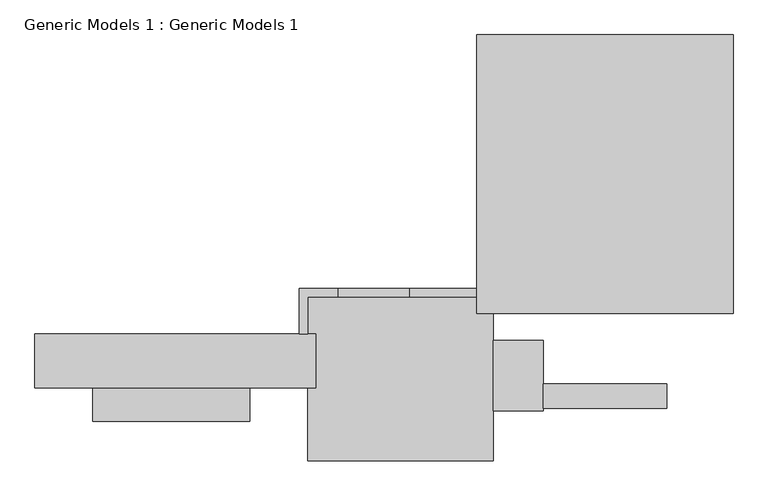
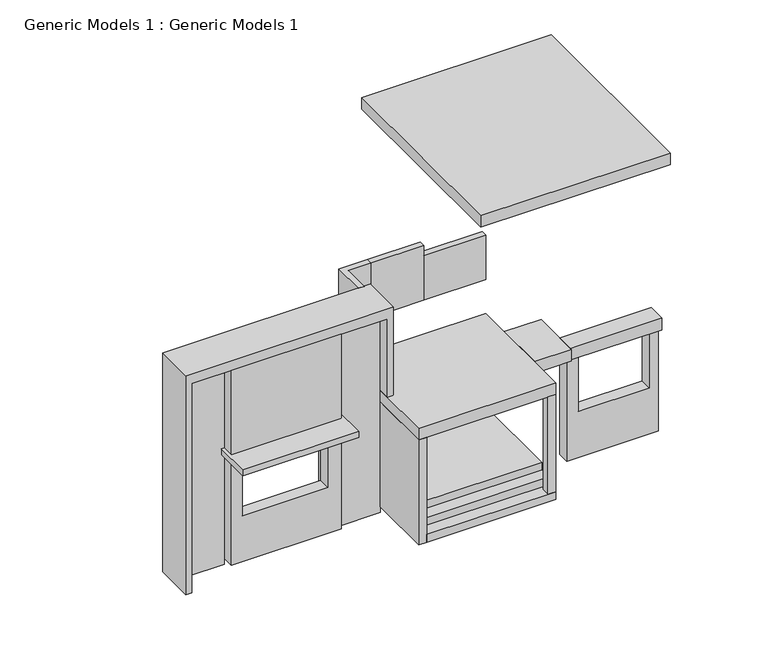
"""IFC4 building model written with IfcOpenShell, lengths in millimetres: proxy geometry, Generic Models 1 : Generic Models 1."""

from ifc_helpers import new_model, si_unit, frame, origin, origin_with_axes, place, context, project, spatial, polyline, outline, extrude, source, transform, mapped, element, save


def generic_models_1_generic_models_1_0fe661e1(model_context):
    return source(origin(), model_context, "Body", "SweptSolid", [
        extrude(outline(polyline([(837.2424957, 4926.6408272), (837.2424957, 2509.0759234), (-2388.5575043, 2509.0759234), (-2388.5575043, 4926.6408272), (837.2424957, 4926.6408272)])), origin_with_axes(), (0.0, 0.0, 1.0), 609.6),
        extrude(outline(polyline([(837.2424957, 2509.0759234), (837.2424957, 2204.2759234), (-2388.5575043, 2204.2759234), (-2388.5575043, 2509.0759234), (837.2424957, 2509.0759234)])), origin_with_axes(), (0.0, 0.0, 1.0), 406.4),
        extrude(outline(polyline([(837.2424957, 2204.2759234), (837.2424957, 1899.4759234), (-2388.5575043, 1899.4759234), (-2388.5575043, 2204.2759234), (837.2424957, 2204.2759234)])), origin_with_axes(), (0.0, 0.0, 1.0), 203.2),
        extrude(outline(polyline([(-2741.0024665, 4240.8408272), (-2741.0024665, 5079.0408272), (-2032.9575043, 5079.0408272), (-2032.9575043, 4926.6408272), (-2591.7575043, 4926.6408272), (-2591.7575043, 4240.8408272), (-2741.0024665, 4240.8408272)])), frame((0.0, 0.0, 3962.4), z_axis=(0.0, 0.0, 1.0), x_axis=(1.0, 0.0, 0.0)), (0.0, 0.0, 1.0), 1442.6857666),
        extrude(outline(polyline([(-3734.7575043, 3250.2408272), (-6477.9575043, 3250.2408272), (-6477.9575043, 3555.0408272), (-3734.7575043, 3555.0408272), (-3734.7575043, 3250.2408272)])), frame((0.0, 0.0, 2921.0), z_axis=(0.0, 0.0, 1.0), x_axis=(1.0, 0.0, 0.0)), (0.0, 0.0, 1.0), 2223.6308899),
        extrude(outline(polyline([(-6477.9575043, 3555.0408272), (-7468.5575043, 3555.0408272), (-7468.5575043, 4240.8408272), (-6477.9575043, 4240.8408272), (-6477.9575043, 3555.0408272)])), frame((0.0, 0.0, -152.4), z_axis=(0.0, 0.0, 1.0), x_axis=(1.0, 0.0, 0.0)), (0.0, 0.0, 1.0), 5297.0308899),
        extrude(outline(polyline([(-2591.7575043, 3555.0408272), (-3734.7575043, 3555.0408272), (-3734.7575043, 4240.8408272), (-2591.7575043, 4240.8408272), (-2591.7575043, 3555.0408272)])), frame((0.0, 0.0, -152.4), z_axis=(0.0, 0.0, 1.0), x_axis=(1.0, 0.0, 0.0)), (0.0, 0.0, 1.0), 5297.0308899),
        extrude(outline(polyline([(-2032.9575043, 4926.6408272), (-2032.9575043, 5079.0408272), (-712.1575043, 5079.0408272), (-712.1575043, 4926.6408272), (-2032.9575043, 4926.6408272)])), frame((0.0, 0.0, 3962.4), z_axis=(0.0, 0.0, 1.0), x_axis=(1.0, 0.0, 0.0)), (0.0, 0.0, 1.0), 1442.6857666),
        extrude(outline(polyline([(-712.1575043, 4926.6408272), (-712.1575043, 5079.0408272), (837.2424957, 5079.0408272), (837.2424957, 4926.6408272), (-712.1575043, 4926.6408272)])), frame((0.0, 0.0, 3962.4), z_axis=(0.0, 0.0, 1.0), x_axis=(1.0, 0.0, 0.0)), (0.0, 0.0, 1.0), 1182.2308899),
        extrude(outline(polyline([(5256.8424957, 9765.3408272), (5256.8424957, 4621.8408272), (532.4424957, 4621.8408272), (532.4424957, 9765.3408272), (5256.8424957, 9765.3408272)])), frame((0.0, 0.0, 5638.8), z_axis=(0.0, 0.0, 1.0), x_axis=(1.0, 0.0, 0.0)), (0.0, 0.0, 1.0), 304.8),
        extrude(outline(polyline([(634.0424957, 1899.4759234), (634.0424957, 2102.6759234), (837.2424957, 2102.6759234), (837.2424957, 1899.4759234), (634.0424957, 1899.4759234)])), origin_with_axes(), (0.0, 0.0, 1.0), 2768.6),
        extrude(outline(polyline([(-2388.5575043, 1899.4759234), (-2591.7575043, 1899.4759234), (-2591.7575043, 4926.6408272), (-2388.5575043, 4926.6408272), (-2388.5575043, 1899.4759234)])), origin_with_axes(), (0.0, 0.0, 1.0), 2768.6),
        extrude(outline(polyline([(-372.9328536, -7468.5575043), (5144.6308899, -7468.5575043), (5144.6308899, -2591.7575043), (3073.4, -2591.7575043), (3073.4, -2439.3575043), (5405.0857666, -2439.3575043), (5405.0857666, -7620.9575043), (-372.9328536, -7620.9575043), (-372.9328536, -7468.5575043)])), frame((0.0, 3250.2408272, 0.0), z_axis=(0.0, 1.0, 0.0), x_axis=(0.0, 0.0, 1.0)), (0.0, 0.0, 1.0), 990.6),
        extrude(outline(polyline([(2768.6, 2043.7424957), (2768.6, 1751.6424957), (0.0, 1751.6424957), (0.0, 4037.6424957), (2768.6, 4037.6424957), (2768.6, 3809.0424957), (1219.2, 3809.0424957), (1219.2, 2043.7424957), (2768.6, 2043.7424957)])), frame((0.0, 3021.6408272, 0.0), z_axis=(0.0, 1.0, 0.0), x_axis=(0.0, 0.0, 1.0)), (0.0, 0.0, 1.0), 304.8),
        extrude(outline(polyline([(4037.6424957, 3326.4408272), (4037.6424957, 2866.1028428), (1751.6424957, 2866.1028428), (1751.6424957, 3326.4408272), (4037.6424957, 3326.4408272)])), frame((0.0, 0.0, 2768.6), z_axis=(0.0, 0.0, 1.0), x_axis=(1.0, 0.0, 0.0)), (0.0, 0.0, 1.0), 307.9830591),
        extrude(outline(polyline([(1751.6424957, 4126.5408272), (1751.6424957, 2823.04984), (837.2424957, 2823.04984), (837.2424957, 4126.5408272), (1751.6424957, 4126.5408272)])), frame((0.0, 0.0, 2768.6), z_axis=(0.0, 0.0, 1.0), x_axis=(1.0, 0.0, 0.0)), (0.0, 0.0, 1.0), 307.9830591),
        extrude(outline(polyline([(837.2424957, 1899.4759234), (-2591.7575043, 1899.4759234), (-2591.7575043, 4926.6408272), (837.2424957, 4926.6408272), (837.2424957, 1899.4759234)])), frame((0.0, 0.0, 2768.6), z_axis=(0.0, 0.0, 1.0), x_axis=(1.0, 0.0, 0.0)), (0.0, 0.0, 1.0), 304.8),
        extrude(outline(polyline([(-3658.5575043, 2632.3348921), (-6554.1575043, 2632.3348921), (-6554.1575043, 3555.0408272), (-3658.5575043, 3555.0408272), (-3658.5575043, 2632.3348921)])), frame((0.0, 0.0, 2768.6), z_axis=(0.0, 0.0, 1.0), x_axis=(1.0, 0.0, 0.0)), (0.0, 0.0, 1.0), 152.4),
        extrude(outline(polyline([(2768.6, -6211.2575043), (2768.6, -6477.9575043), (0.0, -6477.9575043), (0.0, -3734.7575043), (2768.6, -3734.7575043), (2768.6, -4077.6575043), (1219.2, -4077.6575043), (1219.2, -6211.2575043), (2768.6, -6211.2575043)])), frame((0.0, 3250.2408272, 0.0), z_axis=(0.0, 1.0, 0.0), x_axis=(0.0, 0.0, 1.0)), (0.0, 0.0, 1.0), 304.8),
    ])


if __name__ == "__main__":
    model = new_model("IFC4")
    model_context = context("Model", 3, world=origin())
    ifc_project = project(units=[si_unit("LENGTHUNIT", "METRE", prefix="MILLI")], contexts=[model_context])
    site = spatial("IfcSite", under=ifc_project)
    building = spatial("IfcBuilding", under=site)
    placement = place(None, origin())
    generic_models_1_generic_models_1_shape = generic_models_1_generic_models_1_0fe661e1(model_context)
    element("IfcBuildingElementProxy", 1, Name="Generic Models 1 : Generic Models 1", ObjectType="Generic Models 1 : Generic Models 1", at=placement, inside=building, context=model_context, shape_type="MappedRepresentation", body=[
        mapped(generic_models_1_generic_models_1_shape, transform((0.0, 0.0, 0.0), x_axis=(1.0, 0.0, 0.0), y_axis=(0.0, 1.0, 0.0), z_axis=(0.0, 0.0, 1.0))),
    ])
    save(model, "model.ifc")

# Revit data of these elements
# Element 1 (IfcBuildingElementProxy, "Generic Models 1 : Generic Models 1")
#   Materials on its faces: "Gypsum Wall Board", "Grass", "wood"
# Materials
#   "Gypsum Wall Board": class "Generic", colour RGB 127 127 127, transparency 0, Description = "Gypsum Wall Board", Cost = 0
#   "Grass": class "Generic", colour RGB 104 137 66, transparency 0, Description = "Physical material.", Cost = 0
#   "wood": class "Generic", colour RGB 120 120 120, transparency 0, Cost = 0
